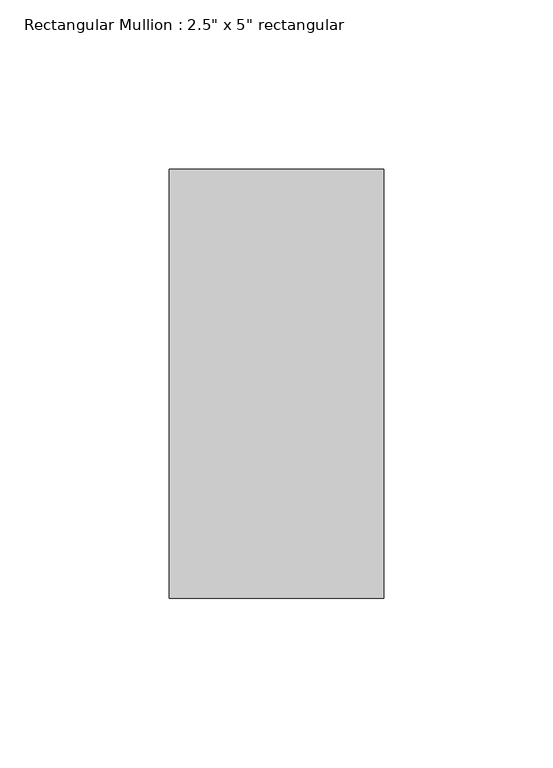
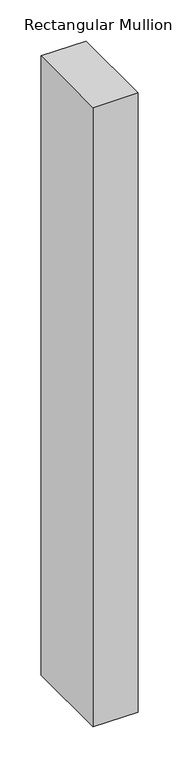
"""IFC4 building model written with IfcOpenShell, lengths in millimetres: member geometry."""

from ifc_helpers import new_model, si_unit, frame, origin, place, context, project, spatial, polyline, outline, extrude, source, transform, mapped, element, save


def member_ff82125d(model_context):
    return source(origin(), model_context, "Body", "SweptSolid", [
        extrude(outline(polyline([(0.0, 63.5), (0.0, -63.5), (-63.5, -63.5), (-63.5, 63.5), (0.0, 63.5)])), frame((0.0, 0.0, -920.75), z_axis=(0.0, 0.0, 1.0), x_axis=(1.0, 0.0, 0.0)), (0.0, 0.0, 1.0), 920.75),
    ])


if __name__ == "__main__":
    model = new_model("IFC4")
    model_context = context("Model", 3, world=origin())
    ifc_project = project(units=[si_unit("LENGTHUNIT", "METRE", prefix="MILLI")], contexts=[model_context])
    site = spatial("IfcSite", under=ifc_project)
    building = spatial("IfcBuilding", under=site)
    placement = place(None, origin())
    member_shape = member_ff82125d(model_context)
    element("IfcMember", 1, ObjectType="Rectangular Mullion : 2.5\" x 5\" rectangular", at=placement, inside=building, context=model_context, shape_type="MappedRepresentation", body=[
        mapped(member_shape, transform((0.0, 0.0, 0.0), x_axis=(1.0, 0.0, 0.0), y_axis=(0.0, 1.0, 0.0), z_axis=(0.0, 0.0, 1.0))),
    ])
    save(model, "model.ifc")

# Revit data of these elements
# Type "Rectangular Mullion : 2.5\" x 5\" rectangular"
#   built-in parameter 1007304 = 0.416667 (stored number, unit not read)
#   built-in parameter 1007301 = 0.104167 (stored number, unit not read)
#   built-in parameter 1007300 = 0.104167 (stored number, unit not read)
# Element 1 (IfcMember, "Rectangular Mullion : 2.5\" x 5\" rectangular")
#   Materials on its faces: "Rectangle 1 sq"
# Materials
#   "Rectangle 1 sq": class "Generic", colour RGB 120 120 120, transparency 0, Cost = 0
